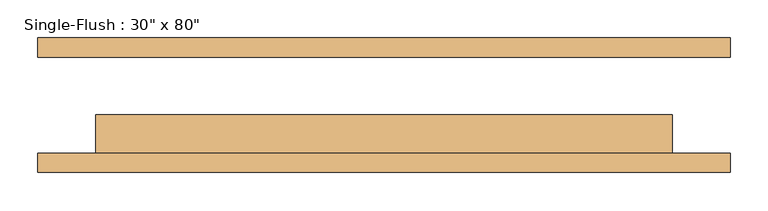
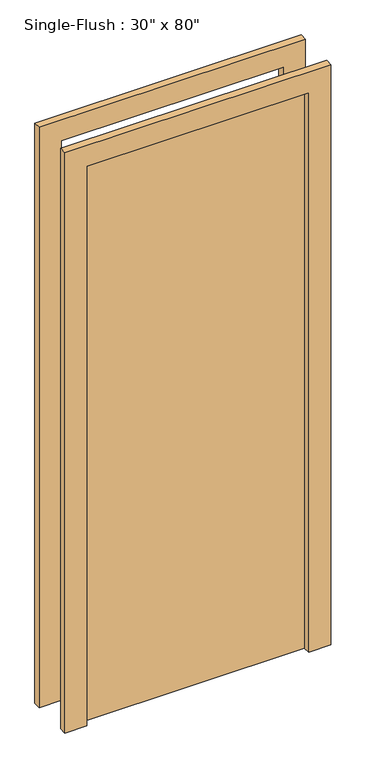
"""IFC4 building model written with IfcOpenShell, lengths in millimetres: door geometry."""

from ifc_helpers import new_model, si_unit, frame, origin, origin_with_axes, place, context, project, spatial, polyline, outline, extrude, source, transform, mapped, element, save


def door_e00f436c(model_context):
    return source(origin(), model_context, "Body", "SweptSolid", [
        extrude(outline(polyline([(2108.2, -457.2), (0.0, -457.2), (0.0, -381.0), (2032.0, -381.0), (2032.0, 381.0), (0.0, 381.0), (0.0, 457.2), (2108.2, 457.2), (2108.2, -457.2)])), frame((0.0, -88.9, 0.0), z_axis=(0.0, 1.0, 0.0), x_axis=(0.0, 0.0, 1.0)), (0.0, 0.0, 1.0), 25.4),
        extrude(outline(polyline([(2108.2, 457.2), (2108.2, -457.2), (0.0, -457.2), (0.0, -381.0), (2032.0, -381.0), (2032.0, 381.0), (0.0, 381.0), (0.0, 457.2), (2108.2, 457.2)])), frame((0.0, 63.5, 0.0), z_axis=(0.0, 1.0, 0.0), x_axis=(0.0, 0.0, 1.0)), (0.0, 0.0, 1.0), 25.4),
        extrude(outline(polyline([(381.0, -12.7), (381.0, -63.5), (-381.0, -63.5), (-381.0, -12.7), (381.0, -12.7)])), origin_with_axes(), (0.0, 0.0, 1.0), 2032.0),
    ])


if __name__ == "__main__":
    model = new_model("IFC4")
    model_context = context("Model", 3, world=origin())
    ifc_project = project(units=[si_unit("LENGTHUNIT", "METRE", prefix="MILLI")], contexts=[model_context])
    site = spatial("IfcSite", under=ifc_project)
    building = spatial("IfcBuilding", under=site)
    placement = place(None, origin())
    door_shape = door_e00f436c(model_context)
    element("IfcDoor", 1, ObjectType="Single-Flush : 30\" x 80\"", at=placement, inside=building, context=model_context, shape_type="MappedRepresentation", body=[
        mapped(door_shape, transform((0.0, 0.0, 0.0), x_axis=(1.0, 0.0, 0.0), y_axis=(0.0, 1.0, 0.0), z_axis=(0.0, 0.0, 1.0))),
    ])
    save(model, "model.ifc")

# Revit data of these elements
# Type "Single-Flush : 30\" x 80\""
#   Type Mark = "5"
#   Construction Type Id = "MDOOR"
#   Assembly Code = "C1020"
#   Analytic Construction = "Metal"
#   Thickness = 0' - 2"
#   Heat Transfer Coefficient (U) = 0.651978 BTU/(h·ft²·°F)
#   Height = 6' - 8"
#   Trim Projection Ext = 0' - 1"
#   Trim Projection Int = 0' - 1"
#   Trim Width = 0' - 3"
#   Width = 2' - 6"
#   Define Thermal Properties by = 1
#   Define Thermal Properties by = 1
#   Door Material = Door - Panel
#   Frame Material = Door - Frame
#   Visual Light Transmittance = 0
#   Solar Heat Gain Coefficient = 0
#   Function = (empty or 0)
#   Wall Closure = (empty or 0)
# Element 1 (IfcDoor, "Single-Flush : 30\" x 80\"")
#   Materials on its faces: "Door - Frame", "Door - Panel"
# Materials
#   "Door - Panel": class "Wood", colour RGB 210 159 95, transparency 0, Cost = 0
#   "Door - Frame": colour RGB 118 70 51, transparency 0, Cost = 0
